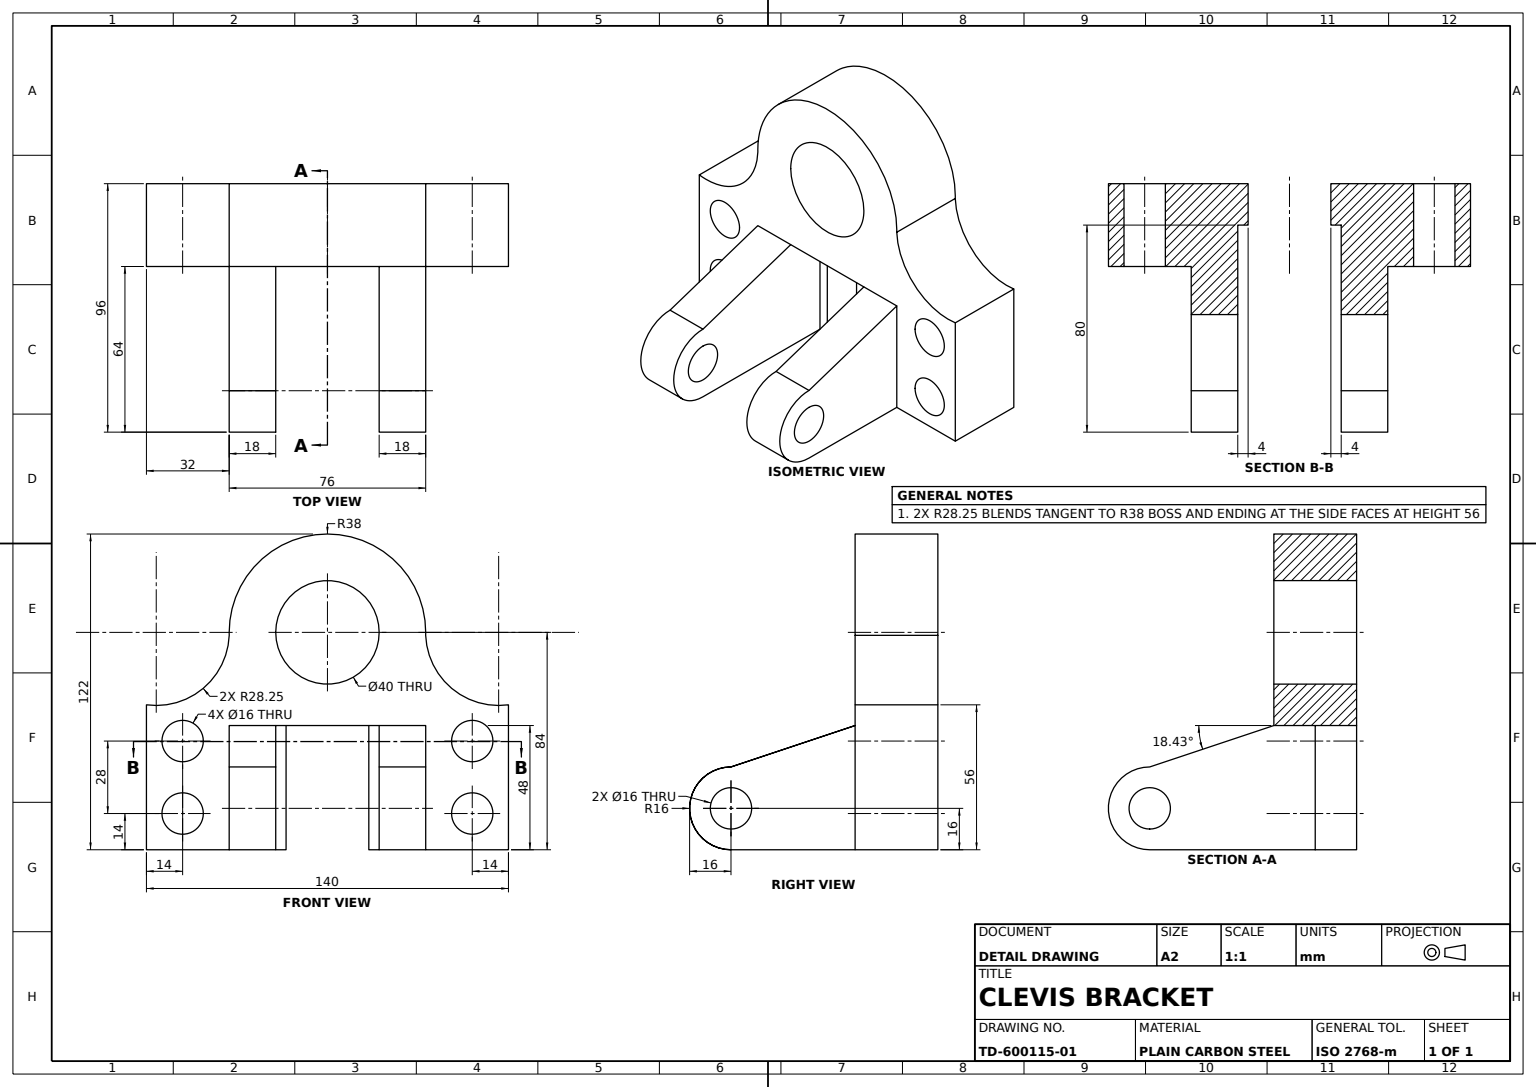
from build123d import *
from build123d.topology import SkipClean

# Parameters (mm, degrees)
BRACKET_MASTER_PROFILE_SKETCH_R   = 8
BRACKET_MASTER_PROFILE_SKETCH_R_2 = 20
BASE_BLOCK_32MM_DEPTH             = 16
SKETCH1_5_W                       = 18
SKETCH1_5_H                       = 48
BORE_BOSS_BODY_64MM_DEPTH         = 64
CLEVIS_LUGS_76MM_DEPTH            = 76
LUG_PROFILE_CUT_A_DEPTH           = 142
LUG_PROFILE_CUT_B_DEPTH           = 142
SKETCH1_6_W                       = 32
SKETCH1_6_H                       = 48
PROFILE_CUT_131MM_DEPTH           = 131
SKETCH1_7_W                       = 18
SKETCH1_7_H                       = 48
PROFILE_BOSS_16MM_DEPTH           = 16
SKETCH1_15_W                      = 4
SKETCH1_15_H                      = 48
PROFILE_BOSS_32MM_DEPTH           = 16
SKETCH1_16_W                      = 4
SKETCH1_16_H                      = 48
THROUGH_CUT_147MM_DEPTH           = 147


with BuildPart() as part:
    # Bracket Master Profile Sketch → Base Block 32mm (new, symmetric)
    with BuildSketch(Plane.XY):
        with BuildLine():
            Line((-70, 56), (-70, 0))
            Line((-70, 0), (-38, 0))
            Line((-38, 0), (-38, 48))
            Line((-38, 48), (-20, 48))
            Line((-20, 48), (-16, 48))
            Line((-16, 48), (16, 48))
            Line((16, 48), (20, 48))
            Line((20, 48), (38, 48))
            Line((38, 48), (38, 0))
            Line((38, 0), (70, 0))
            Line((70, 0), (70, 56))
            ThreePointArc((70, 56), (48.056901395, 62.34853625), (37.98259606, 82.850044997))
            ThreePointArc((37.98259606, 82.850044997), (0, 122), (-37.98259606, 82.850044997))
            ThreePointArc((-37.98259606, 82.850044997), (-48.056901395, 62.34853625), (-70, 56))
        make_face()
        with Locations((-56, 14)):
            Circle(BRACKET_MASTER_PROFILE_SKETCH_R, mode=Mode.SUBTRACT)
        with Locations((-56, 42)):
            Circle(BRACKET_MASTER_PROFILE_SKETCH_R, mode=Mode.SUBTRACT)
        with Locations((56, 14)):
            Circle(BRACKET_MASTER_PROFILE_SKETCH_R, mode=Mode.SUBTRACT)
        with Locations((56, 42)):
            Circle(BRACKET_MASTER_PROFILE_SKETCH_R, mode=Mode.SUBTRACT)
        with Locations((0, 84)):
            Circle(BRACKET_MASTER_PROFILE_SKETCH_R_2, mode=Mode.SUBTRACT)
    extrude(amount=BASE_BLOCK_32MM_DEPTH, both=True)

    # Sketch1_5 → Bore Boss Body 64mm (add)
    with BuildSketch(Plane.XY):
        with Locations((-29, 24)):
            Rectangle(SKETCH1_5_W, SKETCH1_5_H)
        with Locations((29, 24)):
            Rectangle(SKETCH1_5_W, SKETCH1_5_H)
    extrude(amount=BORE_BOSS_BODY_64MM_DEPTH)

    # Clevis Lug Profile Sketch → Clevis Lugs 76mm (add)
    with BuildSketch(Plane.ZY.offset(38)):
        with BuildLine():
            ThreePointArc((64, 32), (48, 16), (64, 0))
            Line((64, 0), (64, 8))
            ThreePointArc((64, 8), (56, 16), (64, 24))
            Line((64, 24), (64, 32))
        make_face()
        with BuildLine():
            Line((64, 8), (64, 0))
            ThreePointArc((64, 0), (75.313708499, 4.686291501), (80, 16))
            ThreePointArc((80, 16), (75.313708499, 27.313708499), (64, 32))
            Line((64, 32), (64, 24))
            ThreePointArc((64, 24), (69.656854249, 21.656854249), (72, 16))
            ThreePointArc((72, 16), (69.656854249, 10.343145751), (64, 8))
        make_face()
        with BuildLine():
            ThreePointArc((64, 32), (48, 16), (64, 0))
            Line((64, 0), (64, 8))
            ThreePointArc((64, 8), (56, 16), (64, 24))
            Line((64, 24), (64, 32))
        make_face()
        with BuildLine():
            Line((64, 8), (64, 0))
            ThreePointArc((64, 0), (75.313708499, 4.686291501), (80, 16))
            ThreePointArc((80, 16), (75.313708499, 27.313708499), (64, 32))
            Line((64, 32), (64, 24))
            ThreePointArc((64, 24), (69.656854249, 21.656854249), (72, 16))
            ThreePointArc((72, 16), (69.656854249, 10.343145751), (64, 8))
        make_face()
    extrude(amount=-CLEVIS_LUGS_76MM_DEPTH)

    # Sketch2_3 → Lug Profile Cut A (cut)
    with SkipClean():  # the faces are left unmerged after this step: merging them gives an invalid solid
        with BuildSketch(Plane.ZY.offset(38)):
            with BuildLine():
                ThreePointArc((64, 24), (56, 16), (64, 8))
                Line((64, 8), (64, 16))
                Line((64, 16), (64, 24))
            make_face()
            with BuildLine():
                Line((64, 16), (64, 8))
                ThreePointArc((64, 8), (69.656854249, 10.343145751), (72, 16))
                ThreePointArc((72, 16), (69.656854249, 21.656854249), (64, 24))
                Line((64, 24), (64, 16))
            make_face()
        extrude(amount=-LUG_PROFILE_CUT_A_DEPTH, mode=Mode.SUBTRACT)

    # Sketch2_4 → Lug Profile Cut B (cut)
    with SkipClean():  # the faces are left unmerged after this step: merging them gives an invalid solid
        with BuildSketch(Plane.ZY.offset(38)):
            Polygon((16, 48), (64, 32), (64, 48), align=None)
        extrude(amount=-LUG_PROFILE_CUT_B_DEPTH, mode=Mode.SUBTRACT)

    # Sketch1_6 → Profile Cut 131mm (cut)
    with SkipClean():  # the faces are left unmerged after this step: merging them gives an invalid solid
        with BuildSketch(Plane.XY):
            with Locations((0, 24)):
                Rectangle(SKETCH1_6_W, SKETCH1_6_H)
        extrude(amount=PROFILE_CUT_131MM_DEPTH, mode=Mode.SUBTRACT)

    # Sketch1_7 → Profile Boss 16mm (add)
    with SkipClean():  # the faces are left unmerged after this step: merging them gives an invalid solid
        with BuildSketch(Plane.XY):
            with Locations((-29, 24)):
                Rectangle(SKETCH1_7_W, SKETCH1_7_H)
            with Locations((29, 24)):
                Rectangle(SKETCH1_7_W, SKETCH1_7_H)
        extrude(amount=-PROFILE_BOSS_16MM_DEPTH)

    # Sketch1_15 → Profile Boss 32mm (add, symmetric)
    with SkipClean():  # the faces are left unmerged after this step: merging them gives an invalid solid
        with BuildSketch(Plane.XY):
            with Locations((-18, 24)):
                Rectangle(SKETCH1_15_W, SKETCH1_15_H)
            with Locations((18, 24)):
                Rectangle(SKETCH1_15_W, SKETCH1_15_H)
        extrude(amount=PROFILE_BOSS_32MM_DEPTH, both=True)

    # Sketch1_16 → Through Cut 147mm (cut)
    with SkipClean():  # the faces are left unmerged after this step: merging them gives an invalid solid
        with BuildSketch(Plane.XY):
            with Locations((-18, 24)):
                Rectangle(SKETCH1_16_W, SKETCH1_16_H)
            with Locations((18, 24)):
                Rectangle(SKETCH1_16_W, SKETCH1_16_H)
        extrude(amount=THROUGH_CUT_147MM_DEPTH, mode=Mode.SUBTRACT)


solid = part.part
